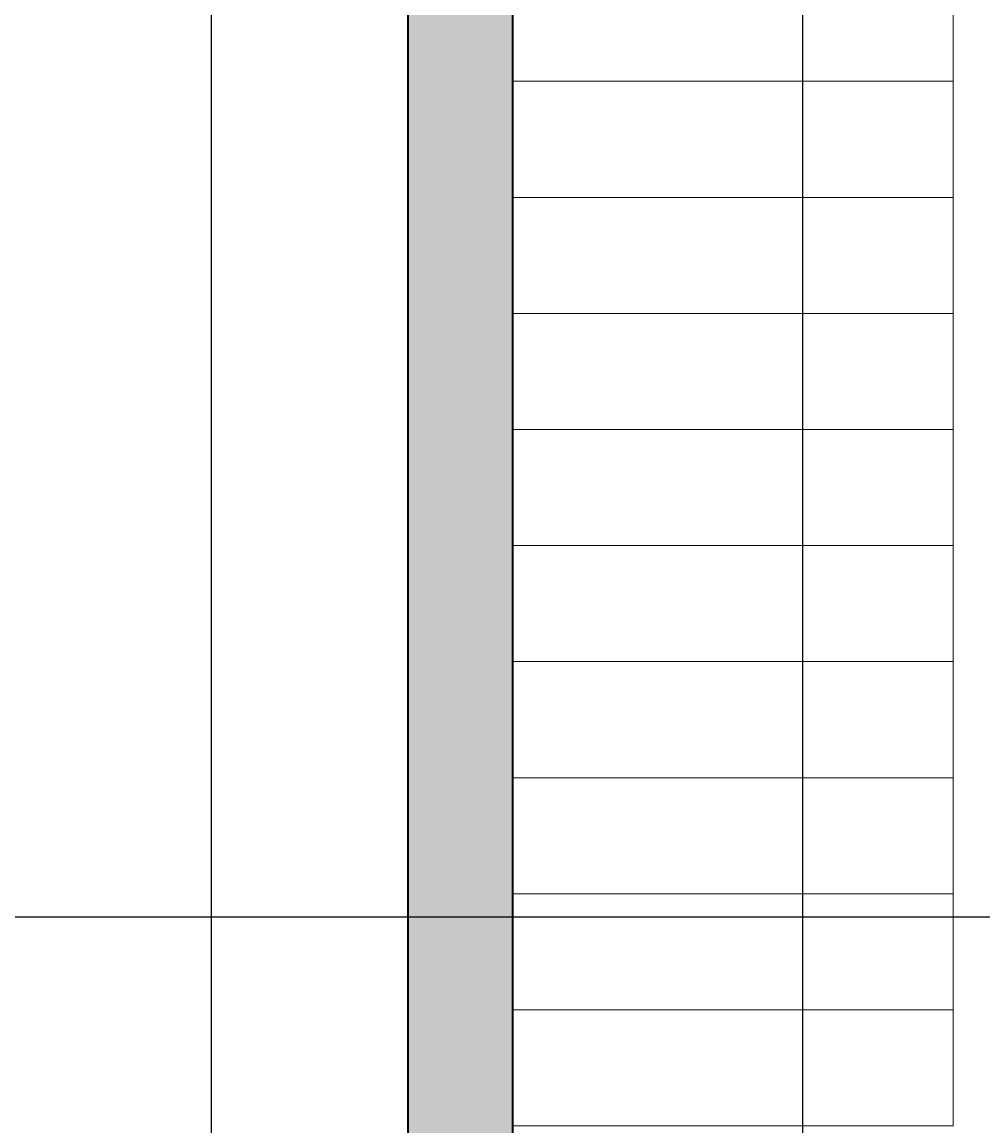
# Model space of a CAD drawing. Units: inches. Extents: x 37 to 706, y -568 to 110.
# Tile 10 of 24: x 361 to 444, y -468 to -373. Entities that reach past the tile are written whole.
import ezdxf

# ---------------------------------------------------------------- set-up
doc = ezdxf.new("R2010")
doc.units = ezdxf.units.IN
doc.header["$MEASUREMENT"] = 0
for name, color, linetype, lineweight in [('A-ANNO-DIMS', 2, 'Continuous', 18), ('A-FLOR-STRS', 7, 'Continuous', 18), ('A-WALL', 7, 'Continuous', 35), ('A-WALL-PATT', 252, 'Continuous', 13)]:
    doc.layers.add(name, color=color, linetype=linetype, lineweight=lineweight)
doc.styles.get("Standard").update_dxf_attribs({"font": 'arial.ttf'})
doc.dimstyles.get("Standard").update_dxf_attribs({"dimtxt": 0.18, "dimasz": 0.18, "dimexe": 0.18, "dimexo": 0.0625, "dimgap": 0.09, "dimtad": 0, "dimtih": 1, "dimtoh": 1, "dimdec": 0, "dimzin": 0, "dimdsep": 46, "dimlunit": 3, "dimtxsty": 'Standard', "dimcen": 0.09, "dimadec": 0, "dimazin": 0, "dimtfac": 1, "dimtdec": 0, "dimtofl": 0, "dimtmove": 0, "dimatfit": 3, "dimfxl": 1, "dimtolj": 1, "dimtzin": 0, "dimarcsym": 0})

# ---------------------------------------------------------------- blocks, each defined once
blk = doc.blocks.new('*D5')
at = {"layer": 'A-ANNO-DIMS', "color": 0, "lineweight": -2, "transparency": 16777216}
for p, q in [((393.896, 51.292), (376.844, 51.292)), ((377.024, 51.112), (377.024, -232.555)), ((377.024, -522.528), (377.024, -238.862)), ((393.896, -522.708), (376.844, -522.708))]:
    blk.add_line(p, q, dxfattribs=at)
at = {"layer": 'A-ANNO-DIMS', "color": 0, "transparency": 16777216}
for points in [[(376.994, 51.112), (377.054, 51.112), (377.024, 51.292)], [(376.994, -522.528), (377.054, -522.528), (377.024, -522.708)]]:
    blk.add_solid(points, dxfattribs=at)
at = {"layer": 'Defpoints', "color": 0, "transparency": 16777216}
for p in [(393.958, 51.292), (377.024, -522.708), (393.958, -522.708)]:
    blk.add_point(p, dxfattribs=at)
at = {"layer": 'A-ANNO-DIMS', "color": 0, "transparency": 16777216, "insert": (377.024, -235.708), "char_height": 6, "attachment_point": 5}
blk.add_mtext('\\A1;47\'-10"', dxfattribs=at)
blk = doc.blocks.new('*D45')
at = {"layer": 'A-ANNO-DIMS', "color": 0, "lineweight": -2, "transparency": 16777216}
for p, q in [((88.021, -449.708), (705.888, -449.708)), ((705.708, -449.888), (705.708, -481.527)), ((705.708, -513.528), (705.708, -481.89)), ((79.021, -513.708), (705.888, -513.708))]:
    blk.add_line(p, q, dxfattribs=at)
at = {"layer": 'A-ANNO-DIMS', "color": 0, "transparency": 16777216}
for points in [[(705.678, -449.888), (705.738, -449.888), (705.708, -449.708)], [(705.678, -513.528), (705.738, -513.528), (705.708, -513.708)]]:
    blk.add_solid(points, dxfattribs=at)
at = {"layer": 'Defpoints', "color": 0, "transparency": 16777216}
for p in [(87.958, -449.708), (705.708, -449.708), (78.958, -513.708)]:
    blk.add_point(p, dxfattribs=at)
at = {"layer": 'A-ANNO-DIMS', "color": 0, "transparency": 16777216, "insert": (705.708, -481.708), "char_height": 0.18, "attachment_point": 5}
blk.add_mtext('\\A1;5\'-4"', dxfattribs=at)
blk = doc.blocks.new('*D56')
at = {"layer": 'A-ANNO-DIMS', "color": 0, "lineweight": -2, "transparency": 16777216}
for p, q in [((402.958, -142.771), (402.958, -567.638)), ((427.967, -142.771), (427.967, -567.638)), ((403.138, -567.458), (415.132, -567.458)), ((427.787, -567.458), (415.794, -567.458))]:
    blk.add_line(p, q, dxfattribs=at)
at = {"layer": 'A-ANNO-DIMS', "color": 0, "transparency": 16777216}
for points in [[(403.138, -567.428), (403.138, -567.488), (402.958, -567.458)], [(427.787, -567.428), (427.787, -567.488), (427.967, -567.458)]]:
    blk.add_solid(points, dxfattribs=at)
at = {"layer": 'Defpoints', "color": 0, "transparency": 16777216}
for p in [(402.958, -142.708), (427.967, -142.708), (427.967, -567.458)]:
    blk.add_point(p, dxfattribs=at)
at = {"layer": 'A-ANNO-DIMS', "color": 0, "transparency": 16777216, "insert": (415.463, -567.458), "char_height": 0.18, "attachment_point": 5}
blk.add_mtext('\\A1;2\'-1"', dxfattribs=at)

msp = doc.modelspace()

# ---------------------------------------------------------------- hatches: boundary and pattern name
at = {"layer": 'A-WALL-PATT'}
h = msp.add_hatch(color=256, dxfattribs=at)
h.dxf.hatch_style = 1
h.paths.add_polyline_path([(220.958, -351.708), (211.958, -351.708), (211.958, -513.708), (254.958, -513.708), (254.958, -504.708), (220.958, -504.708)], flags=17)
h.paths.add_polyline_path([(220.958, -294.708), (211.958, -294.708), (211.958, -303.708), (220.958, -303.708)], flags=17)
h.paths.add_polyline_path([(175.958, -294.708), (155.871, -294.708), (155.871, -303.708), (155.958, -303.708), (175.958, -303.708)], flags=17)
h.paths.add_polyline_path([(220.958, -16.708), (211.958, -16.708), (211.958, -142.708), (220.958, -142.708)], flags=17)
h.paths.add_polyline_path([(357.958, 51.292), (78.958, 51.292), (78.958, -513.708), (87.958, -513.708), (87.958, -303.708), (95.871, -303.708), (95.871, -294.708), (87.958, -294.708), (87.958, -142.708), (187.958, -142.708), (187.958, -133.708), (87.958, -133.708), (87.958, -25.708), (106.958, -25.708), (106.958, -16.708), (87.958, -16.708), (87.958, 42.292), (348.958, 42.292), (348.958, 17.129), (348.958, -133.708), (246.958, -133.708), (246.958, -142.708), (348.958, -142.708), (348.958, -294.708), (251.958, -294.708), (251.958, -303.708), (348.958, -303.708), (348.958, -351.708), (260.958, -351.708), (260.958, -329.708), (251.958, -329.708), (251.958, -360.708), (327.446, -360.708), (348.958, -360.708), (348.958, -504.708), (314.958, -504.708), (314.958, -513.708), (357.958, -513.708)])
h.paths.add_polyline_path([(416.958, -303.708), (402.958, -303.708), (402.958, -151.708), (478.958, -151.708), (478.958, -142.708), (402.958, -142.708), (402.958, -22.708), (409.958, -22.708), (409.958, -13.708), (402.958, -13.708), (402.958, 42.292), (663.958, 42.292), (663.958, -303.708), (566.958, -303.708), (566.958, -312.708), (663.958, -312.708), (663.958, -360.708), (575.958, -360.708), (575.958, -338.708), (566.958, -338.708), (566.958, -360.708), (566.958, -369.708), (642.446, -369.708), (663.958, -369.708), (663.958, -513.708), (629.958, -513.708), (629.958, -522.708), (672.958, -522.708), (672.958, 51.292), (393.958, 51.292), (393.958, -522.708), (402.958, -522.708), (402.958, -312.708), (416.958, -312.708)])
h.paths.add_polyline_path([(490.958, -303.708), (476.958, -303.708), (476.958, -312.708), (490.958, -312.708)], flags=17)
h.paths.add_polyline_path([(535.958, -303.708), (526.958, -303.708), (526.958, -312.708), (535.958, -312.708)], flags=17)
h.paths.add_polyline_path([(535.958, -369.708), (526.958, -369.708), (526.958, -522.708), (569.958, -522.708), (569.958, -513.708), (535.958, -513.708)], flags=17)
h.paths.add_polyline_path([(511.958, -13.708), (502.958, -13.708), (502.958, -151.708), (511.958, -151.708)], flags=17)
h.paths.add_polyline_path([(651.539, -142.708), (651.539, -120.181), (642.539, -120.181), (642.539, -142.708), (550.539, -142.708), (550.539, -120.708), (541.539, -120.708), (541.539, -142.708), (537.958, -142.708), (537.958, -151.708), (651.539, -151.708)], flags=17)
h.paths.add_polyline_path([(651.539, -85.708), (541.539, -85.708), (541.539, -94.708), (651.539, -94.708)], flags=17)
h.paths.add_polyline_path([(476.958, -13.708), (469.958, -13.708), (469.958, -22.708), (476.958, -22.708)], flags=17)
h.paths.add_polyline_path([(185.958, -16.708), (166.958, -16.708), (166.958, -25.708), (185.958, -25.708)], flags=17)
h.paths.add_polyline_path([(168.909, -414.719), (214.621, -414.719), (214.621, -392.33), (168.909, -392.33)], flags=25)

# ---------------------------------------------------------------- linework, layer by layer
at = {"layer": 'A-FLOR-STRS'}
for p, q in [((440.958, -357.708), (440.958, -467.708)), ((440.958, -377.708), (402.958, -377.708)), ((440.958, -387.708), (402.958, -387.708)), ((440.958, -397.708), (402.958, -397.708)), ((440.958, -407.708), (402.958, -407.708)), ((440.958, -417.708), (402.958, -417.708)), ((440.958, -427.708), (402.958, -427.708)), ((440.958, -437.708), (402.958, -437.708)), ((440.958, -447.708), (402.958, -447.708)), ((440.958, -457.708), (402.958, -457.708)), ((440.958, -467.708), (402.958, -467.708))]:
    msp.add_line(p, q, dxfattribs=at)
at = {"layer": 'A-WALL'}
for p, q in [((393.958, 51.292), (393.958, -522.708)), ((402.958, -312.708), (402.958, -522.708))]:
    msp.add_line(p, q, dxfattribs=at)

# ---------------------------------------------------------------- dimensions: what is measured, and where the dimension line sits
at = {"layer": 'A-ANNO-DIMS'}
for base, p1, p2, override, picture, middle in [((377.024, -522.708), (393.958, 51.292), (393.958, -522.708), {"dimtxt": 6, "dimclrd": 0, "dimclre": 0, "dimclrt": 0}, '*D5', (377.024, -235.708)), ((705.708, -449.708), (78.958, -513.708), (87.958, -449.708), {"dimdec": 1, "dimlfac": 1, "dimrnd": 0, "dimzin": 1, "dimdsep": 46, "dimlunit": 4, "dimfrac": 2}, '*D45', (705.708, -481.708))]:
    dim = msp.add_linear_dim(base=base, p1=p1, p2=p2, angle=90, dimstyle='Standard', override=override, dxfattribs=at)
    dim.commit()
    dim.dimension.update_dxf_attribs({"geometry": picture, "text_midpoint": middle})
dim = msp.add_linear_dim(base=(427.967, -567.458), p1=(402.958, -142.708), p2=(427.967, -142.708), dimstyle='Standard', override={"dimdec": 1, "dimlfac": 1, "dimrnd": 0, "dimzin": 1, "dimdsep": 46, "dimlunit": 4, "dimfrac": 2}, dxfattribs=at)
dim.commit()
dim.dimension.update_dxf_attribs({"geometry": '*D56', "text_midpoint": (415.463, -567.458)})

doc.saveas('drawing.dxf')
